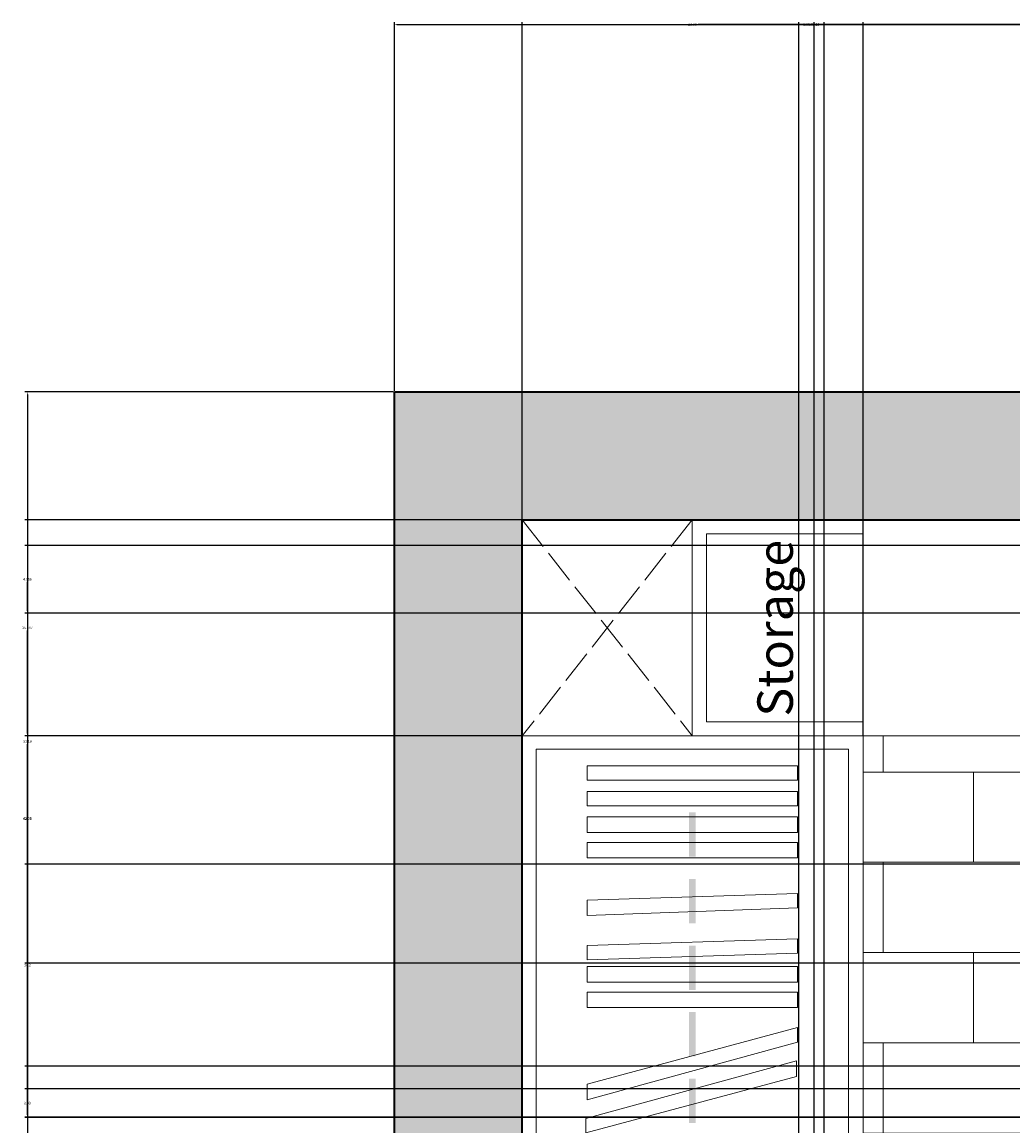
# Model space of a CAD drawing. Units: inches. Extents: x 6 to 575, y 34 to 566.
# Tile 8 of 21: x 6 to 76, y 488 to 566. Entities that reach past the tile are written whole.
import ezdxf

# ---------------------------------------------------------------- set-up
doc = ezdxf.new("R2010")
doc.units = ezdxf.units.IN
doc.linetypes.add('ACAD_ISO02W100', pattern=[15, 12, -3])
for name, color, linetype, lineweight in [('A-ANNO-DIMS', 2, 'Continuous', 18), ('A-ANNO-TEXT', 6, 'Continuous', 18), ('A-FLOR-CASE', 2, 'Continuous', 18), ('A-FLOR-CASE-HIDN', 2, 'ACAD_ISO02W100', 13), ('A-FLOR-PATT', 252, 'Continuous', 9), ('A-WALL-PATT', 251, 'Continuous', 9), ('WALLS', 7, 'Continuous', 35)]:
    doc.layers.add(name, color=color, linetype=linetype, lineweight=lineweight)
doc.styles.add('PDF Century Gothic', font='txt')
doc.styles.get("Standard").update_dxf_attribs({"font": 'arial.ttf'})
doc.dimstyles.get("Standard").update_dxf_attribs({"dimtxt": 0.18, "dimasz": 0.18, "dimexe": 0.18, "dimexo": 0.0625, "dimgap": 0.09, "dimtad": 0, "dimtih": 1, "dimtoh": 1, "dimdec": 4, "dimzin": 0, "dimdsep": 46, "dimtxsty": 'Standard', "dimcen": 0.09, "dimadec": 0, "dimazin": 0, "dimtfac": 1, "dimtdec": 4, "dimtofl": 0, "dimtmove": 0, "dimatfit": 3, "dimfxl": 1, "dimtolj": 1, "dimtzin": 0, "dimarcsym": 0})

# ---------------------------------------------------------------- blocks, each defined once
blk = doc.blocks.new('*D30')
at = {"layer": 'A-ANNO-DIMS', "color": 0, "lineweight": -2, "transparency": 16777216}
for p, q in [((32.596, 539.801), (6.649, 539.801)), ((6.829, 539.621), (6.829, 299.97)), ((6.829, 59.955), (6.829, 299.606)), ((197.625, 59.775), (6.649, 59.775))]:
    blk.add_line(p, q, dxfattribs=at)
at = {"layer": 'A-ANNO-DIMS', "color": 0, "transparency": 16777216}
for points in [[(6.799, 539.621), (6.859, 539.621), (6.829, 539.801)], [(6.799, 59.955), (6.859, 59.955), (6.829, 59.775)]]:
    blk.add_solid(points, dxfattribs=at)
at = {"layer": 'Defpoints', "color": 0, "transparency": 16777216}
for p in [(32.659, 539.801), (6.829, 59.775), (197.687, 59.775)]:
    blk.add_point(p, dxfattribs=at)
at = {"layer": 'A-ANNO-DIMS', "color": 0, "transparency": 16777216, "insert": (6.829, 299.788), "char_height": 0.18, "attachment_point": 5}
blk.add_mtext('\\A1;480', dxfattribs=at)
blk = doc.blocks.new('*D31')
at = {"layer": 'A-ANNO-DIMS', "color": 0, "lineweight": -2, "transparency": 16777216}
for p, q in [((32.659, 539.863), (32.659, 565.811)), ((32.839, 565.631), (96.378, 565.631)), ((160.479, 565.631), (96.939, 565.631)), ((160.659, 539.863), (160.659, 565.811))]:
    blk.add_line(p, q, dxfattribs=at)
at = {"layer": 'A-ANNO-DIMS', "color": 0, "transparency": 16777216}
for points in [[(32.839, 565.661), (32.839, 565.601), (32.659, 565.631)], [(160.479, 565.661), (160.479, 565.601), (160.659, 565.631)]]:
    blk.add_solid(points, dxfattribs=at)
at = {"layer": 'Defpoints', "color": 0, "transparency": 16777216}
for p in [(160.659, 565.631), (32.659, 539.801), (160.659, 539.801)]:
    blk.add_point(p, dxfattribs=at)
at = {"layer": 'A-ANNO-DIMS', "color": 0, "transparency": 16777216, "insert": (96.659, 565.631), "char_height": 0.18, "attachment_point": 5}
blk.add_mtext('\\A1;128', dxfattribs=at)
blk = doc.blocks.new('*D55')
at = {"layer": 'A-ANNO-DIMS', "color": 0, "lineweight": -2, "transparency": 16777216}
for p, q in [((41.659, 286.127), (41.659, 565.811)), ((41.839, 565.631), (81.788, 565.631)), ((122.385, 565.631), (82.436, 565.631)), ((122.565, 286.127), (122.565, 565.811))]:
    blk.add_line(p, q, dxfattribs=at)
at = {"layer": 'A-ANNO-DIMS', "color": 0, "transparency": 16777216}
for points in [[(41.839, 565.661), (41.839, 565.601), (41.659, 565.631)], [(122.385, 565.661), (122.385, 565.601), (122.565, 565.631)]]:
    blk.add_solid(points, dxfattribs=at)
at = {"layer": 'Defpoints', "color": 0, "transparency": 16777216}
for p in [(122.565, 565.631), (41.659, 286.064), (122.565, 286.064)]:
    blk.add_point(p, dxfattribs=at)
at = {"layer": 'A-ANNO-DIMS', "color": 0, "transparency": 16777216, "insert": (82.112, 565.631), "char_height": 0.18, "attachment_point": 5}
blk.add_mtext('\\A1;80.9', dxfattribs=at)
blk = doc.blocks.new('*D66')
at = {"layer": 'A-ANNO-DIMS', "color": 0, "lineweight": -2, "transparency": 16777216}
for p, q in [((41.659, 440.863), (41.659, 565.811)), ((41.839, 565.631), (61.878, 565.631)), ((82.712, 565.631), (62.673, 565.631)), ((82.892, 440.863), (82.892, 565.811))]:
    blk.add_line(p, q, dxfattribs=at)
at = {"layer": 'A-ANNO-DIMS', "color": 0, "transparency": 16777216}
for points in [[(41.839, 565.661), (41.839, 565.601), (41.659, 565.631)], [(82.712, 565.661), (82.712, 565.601), (82.892, 565.631)]]:
    blk.add_solid(points, dxfattribs=at)
at = {"layer": 'Defpoints', "color": 0, "transparency": 16777216}
for p in [(82.892, 565.631), (41.659, 440.801), (82.892, 440.801)]:
    blk.add_point(p, dxfattribs=at)
at = {"layer": 'A-ANNO-DIMS', "color": 0, "transparency": 16777216, "insert": (62.275, 565.631), "char_height": 0.18, "attachment_point": 5}
blk.add_mtext('\\A1;41.23', dxfattribs=at)
blk = doc.blocks.new('*D68')
at = {"layer": 'A-ANNO-DIMS', "color": 0, "lineweight": -2, "transparency": 16777216}
for p, q in [((206.596, 530.801), (6.649, 530.801)), ((6.829, 530.621), (6.829, 509.957)), ((6.829, 488.928), (6.829, 509.593)), ((248.571, 488.748), (6.649, 488.748))]:
    blk.add_line(p, q, dxfattribs=at)
at = {"layer": 'A-ANNO-DIMS', "color": 0, "transparency": 16777216}
for points in [[(6.799, 530.621), (6.859, 530.621), (6.829, 530.801)], [(6.799, 488.928), (6.859, 488.928), (6.829, 488.748)]]:
    blk.add_solid(points, dxfattribs=at)
at = {"layer": 'Defpoints', "color": 0, "transparency": 16777216}
for p in [(206.659, 530.801), (6.829, 488.748), (248.633, 488.748)]:
    blk.add_point(p, dxfattribs=at)
at = {"layer": 'A-ANNO-DIMS', "color": 0, "transparency": 16777216, "insert": (6.829, 509.775), "char_height": 0.18, "attachment_point": 5}
blk.add_mtext('\\A1;42.05', dxfattribs=at)
blk = doc.blocks.new('*D71')
at = {"layer": 'A-ANNO-DIMS', "color": 0, "lineweight": -2, "transparency": 16777216}
for p, q in [((246.62, 490.777), (6.649, 490.777)), ((6.829, 490.597), (6.829, 489.945)), ((6.829, 488.928), (6.829, 489.581)), ((248.571, 488.748), (6.649, 488.748))]:
    blk.add_line(p, q, dxfattribs=at)
at = {"layer": 'A-ANNO-DIMS', "color": 0, "transparency": 16777216}
for points in [[(6.799, 490.597), (6.859, 490.597), (6.829, 490.777)], [(6.799, 488.928), (6.859, 488.928), (6.829, 488.748)]]:
    blk.add_solid(points, dxfattribs=at)
at = {"layer": 'Defpoints', "color": 0, "transparency": 16777216}
for p in [(246.683, 490.777), (6.829, 488.748), (248.633, 488.748)]:
    blk.add_point(p, dxfattribs=at)
at = {"layer": 'A-ANNO-DIMS', "color": 0, "transparency": 16777216, "insert": (6.829, 489.763), "char_height": 0.18, "attachment_point": 5}
blk.add_mtext('\\A1;2.03', dxfattribs=at)
blk = doc.blocks.new('*D111')
at = {"layer": 'A-ANNO-DIMS', "color": 0, "lineweight": -2, "transparency": 16777216}
for p, q in [((41.659, 530.863), (41.659, 565.811)), ((41.839, 565.631), (53.259, 565.631)), ((65.469, 565.631), (54.049, 565.631)), ((65.649, 515.657), (65.649, 565.811))]:
    blk.add_line(p, q, dxfattribs=at)
at = {"layer": 'A-ANNO-DIMS', "color": 0, "transparency": 16777216}
for points in [[(41.839, 565.661), (41.839, 565.601), (41.659, 565.631)], [(65.469, 565.661), (65.469, 565.601), (65.649, 565.631)]]:
    blk.add_solid(points, dxfattribs=at)
at = {"layer": 'Defpoints', "color": 0, "transparency": 16777216}
for p in [(65.649, 565.631), (41.659, 530.801), (65.649, 515.594)]:
    blk.add_point(p, dxfattribs=at)
at = {"layer": 'A-ANNO-DIMS', "color": 0, "transparency": 16777216, "insert": (53.654, 565.631), "char_height": 0.18, "attachment_point": 5}
blk.add_mtext('\\A1;23.99', dxfattribs=at)
blk = doc.blocks.new('*D112')
at = {"layer": 'A-ANNO-DIMS', "color": 0, "lineweight": -2, "transparency": 16777216}
for p, q in [((41.596, 530.801), (6.649, 530.801)), ((6.829, 530.621), (6.829, 523.379)), ((6.829, 515.774), (6.829, 523.016)), ((41.596, 515.594), (6.649, 515.594))]:
    blk.add_line(p, q, dxfattribs=at)
at = {"layer": 'A-ANNO-DIMS', "color": 0, "transparency": 16777216}
for points in [[(6.799, 530.621), (6.859, 530.621), (6.829, 530.801)], [(6.799, 515.774), (6.859, 515.774), (6.829, 515.594)]]:
    blk.add_solid(points, dxfattribs=at)
at = {"layer": 'Defpoints', "color": 0, "transparency": 16777216}
for p in [(41.659, 530.801), (6.829, 515.594), (41.659, 515.594)]:
    blk.add_point(p, dxfattribs=at)
at = {"layer": 'A-ANNO-DIMS', "color": 0, "transparency": 16777216, "insert": (6.829, 523.198), "char_height": 0.18, "attachment_point": 5}
blk.add_mtext('\\A1;15.207', dxfattribs=at)
blk = doc.blocks.new('*D113')
at = {"layer": 'A-ANNO-DIMS', "color": 0, "lineweight": -2, "transparency": 16777216}
for p, q in [((65.649, 530.863), (65.649, 565.811)), ((65.829, 565.631), (91.278, 565.631)), ((117.479, 565.631), (92.03, 565.631)), ((117.659, 530.863), (117.659, 565.811))]:
    blk.add_line(p, q, dxfattribs=at)
at = {"layer": 'A-ANNO-DIMS', "color": 0, "transparency": 16777216}
for points in [[(65.829, 565.661), (65.829, 565.601), (65.649, 565.631)], [(117.479, 565.661), (117.479, 565.601), (117.659, 565.631)]]:
    blk.add_solid(points, dxfattribs=at)
at = {"layer": 'Defpoints', "color": 0, "transparency": 16777216}
for p in [(117.659, 565.631), (65.649, 530.801), (117.659, 530.801)]:
    blk.add_point(p, dxfattribs=at)
at = {"layer": 'A-ANNO-DIMS', "color": 0, "transparency": 16777216, "insert": (91.654, 565.631), "char_height": 0.18, "attachment_point": 5}
blk.add_mtext('\\A1;52.01', dxfattribs=at)
blk = doc.blocks.new('*D115')
at = {"layer": 'A-ANNO-DIMS', "color": 0, "lineweight": -2, "transparency": 16777216}
for p, q in [((60.944, 565.631), (60.764, 565.631)), ((61.124, 427.26), (61.124, 565.811)), ((62.217, 427.26), (62.217, 565.811)), ((62.397, 565.631), (62.577, 565.631))]:
    blk.add_line(p, q, dxfattribs=at)
at = {"layer": 'A-ANNO-DIMS', "color": 0, "transparency": 16777216}
for points in [[(60.944, 565.661), (60.944, 565.601), (61.124, 565.631)], [(62.397, 565.661), (62.397, 565.601), (62.217, 565.631)]]:
    blk.add_solid(points, dxfattribs=at)
at = {"layer": 'Defpoints', "color": 0, "transparency": 16777216}
for p in [(62.217, 565.631), (61.124, 427.198), (62.217, 427.198)]:
    blk.add_point(p, dxfattribs=at)
at = {"layer": 'A-ANNO-DIMS', "color": 0, "transparency": 16777216, "insert": (61.67, 565.631), "char_height": 0.18, "attachment_point": 5}
blk.add_mtext('\\A1;1.09', dxfattribs=at)
blk = doc.blocks.new('*D116')
at = {"layer": 'A-ANNO-DIMS', "color": 0, "lineweight": -2, "transparency": 16777216}
for p, q in [((61.124, 427.26), (61.124, 565.811)), ((61.304, 565.631), (61.706, 565.631)), ((62.739, 565.631), (62.337, 565.631)), ((62.919, 427.26), (62.919, 565.811))]:
    blk.add_line(p, q, dxfattribs=at)
at = {"layer": 'A-ANNO-DIMS', "color": 0, "transparency": 16777216}
for points in [[(61.304, 565.661), (61.304, 565.601), (61.124, 565.631)], [(62.739, 565.661), (62.739, 565.601), (62.919, 565.631)]]:
    blk.add_solid(points, dxfattribs=at)
at = {"layer": 'Defpoints', "color": 0, "transparency": 16777216}
for p in [(62.919, 565.631), (61.124, 427.198), (62.919, 427.198)]:
    blk.add_point(p, dxfattribs=at)
at = {"layer": 'A-ANNO-DIMS', "color": 0, "transparency": 16777216, "insert": (62.022, 565.631), "char_height": 0.18, "attachment_point": 5}
blk.add_mtext('\\A1;1.79', dxfattribs=at)
blk = doc.blocks.new('*D117')
at = {"layer": 'A-ANNO-DIMS', "color": 0, "lineweight": -2, "transparency": 16777216}
for p, q in [((41.596, 515.594), (6.649, 515.594)), ((6.829, 515.414), (6.829, 478.379)), ((6.829, 440.981), (6.829, 478.016)), ((41.596, 440.801), (6.649, 440.801))]:
    blk.add_line(p, q, dxfattribs=at)
at = {"layer": 'A-ANNO-DIMS', "color": 0, "transparency": 16777216}
for points in [[(6.799, 515.414), (6.859, 515.414), (6.829, 515.594)], [(6.799, 440.981), (6.859, 440.981), (6.829, 440.801)]]:
    blk.add_solid(points, dxfattribs=at)
at = {"layer": 'Defpoints', "color": 0, "transparency": 16777216}
for p in [(6.829, 515.594), (41.659, 515.594), (41.659, 440.801)]:
    blk.add_point(p, dxfattribs=at)
at = {"layer": 'A-ANNO-DIMS', "color": 0, "transparency": 16777216, "insert": (6.829, 478.198), "char_height": 0.18, "attachment_point": 5}
blk.add_mtext('\\A1;74.8', dxfattribs=at)
blk = doc.blocks.new('*D118')
at = {"layer": 'A-ANNO-DIMS', "color": 0, "lineweight": -2, "transparency": 16777216}
for p, q in [((65.649, 515.657), (65.649, 565.811)), ((65.829, 565.631), (78.186, 565.631)), ((91.474, 565.631), (79.118, 565.631)), ((91.654, 515.657), (91.654, 565.811))]:
    blk.add_line(p, q, dxfattribs=at)
at = {"layer": 'A-ANNO-DIMS', "color": 0, "transparency": 16777216}
for points in [[(65.829, 565.661), (65.829, 565.601), (65.649, 565.631)], [(91.474, 565.661), (91.474, 565.601), (91.654, 565.631)]]:
    blk.add_solid(points, dxfattribs=at)
at = {"layer": 'Defpoints', "color": 0, "transparency": 16777216}
for p in [(91.654, 565.631), (65.649, 515.594), (91.654, 515.594)]:
    blk.add_point(p, dxfattribs=at)
at = {"layer": 'A-ANNO-DIMS', "color": 0, "transparency": 16777216, "insert": (78.652, 565.631), "char_height": 0.18, "attachment_point": 5}
blk.add_mtext('\\A1;26.005', dxfattribs=at)
blk = doc.blocks.new('*D176')
at = {"layer": 'A-ANNO-DIMS', "color": 0, "lineweight": -2, "transparency": 16777216}
for p, q in [((121.596, 530.801), (6.649, 530.801)), ((6.829, 530.621), (6.829, 509.974)), ((6.829, 488.963), (6.829, 509.61)), ((121.839, 488.783), (6.649, 488.783))]:
    blk.add_line(p, q, dxfattribs=at)
at = {"layer": 'A-ANNO-DIMS', "color": 0, "transparency": 16777216}
for points in [[(6.799, 530.621), (6.859, 530.621), (6.829, 530.801)], [(6.799, 488.963), (6.859, 488.963), (6.829, 488.783)]]:
    blk.add_solid(points, dxfattribs=at)
at = {"layer": 'Defpoints', "color": 0, "transparency": 16777216}
for p in [(121.659, 530.801), (6.829, 488.783), (121.902, 488.783)]:
    blk.add_point(p, dxfattribs=at)
at = {"layer": 'A-ANNO-DIMS', "color": 0, "transparency": 16777216, "insert": (6.829, 509.792), "char_height": 0.18, "attachment_point": 5}
blk.add_mtext('\\A1;42.02', dxfattribs=at)
blk = doc.blocks.new('*D177')
at = {"layer": 'A-ANNO-DIMS', "color": 0, "lineweight": -2, "transparency": 16777216}
for p, q in [((139.252, 528.983), (6.649, 528.983)), ((6.829, 528.803), (6.829, 526.786)), ((6.829, 524.404), (6.829, 526.422)), ((139.252, 524.224), (6.649, 524.224))]:
    blk.add_line(p, q, dxfattribs=at)
at = {"layer": 'A-ANNO-DIMS', "color": 0, "transparency": 16777216}
for points in [[(6.799, 528.803), (6.859, 528.803), (6.829, 528.983)], [(6.799, 524.404), (6.859, 524.404), (6.829, 524.224)]]:
    blk.add_solid(points, dxfattribs=at)
at = {"layer": 'Defpoints', "color": 0, "transparency": 16777216}
for p in [(139.314, 528.983), (6.829, 524.224), (139.314, 524.224)]:
    blk.add_point(p, dxfattribs=at)
at = {"layer": 'A-ANNO-DIMS', "color": 0, "transparency": 16777216, "insert": (6.829, 526.604), "char_height": 0.18, "attachment_point": 5}
blk.add_mtext('\\A1;4.759', dxfattribs=at)
blk = doc.blocks.new('*D181')
at = {"layer": 'A-ANNO-DIMS', "color": 0, "lineweight": -2, "transparency": 16777216}
for p, q in [((197.596, 530.801), (6.649, 530.801)), ((6.829, 530.621), (6.829, 515.387)), ((6.829, 499.788), (6.829, 515.023)), ((170.657, 499.608), (6.649, 499.608))]:
    blk.add_line(p, q, dxfattribs=at)
at = {"layer": 'A-ANNO-DIMS', "color": 0, "transparency": 16777216}
for points in [[(6.799, 530.621), (6.859, 530.621), (6.829, 530.801)], [(6.799, 499.788), (6.859, 499.788), (6.829, 499.608)]]:
    blk.add_solid(points, dxfattribs=at)
at = {"layer": 'Defpoints', "color": 0, "transparency": 16777216}
for p in [(197.659, 530.801), (6.829, 499.608), (170.719, 499.608)]:
    blk.add_point(p, dxfattribs=at)
at = {"layer": 'A-ANNO-DIMS', "color": 0, "transparency": 16777216, "insert": (6.829, 515.205), "char_height": 0.18, "attachment_point": 5}
blk.add_mtext('\\A1;31.19', dxfattribs=at)
blk = doc.blocks.new('*D183')
at = {"layer": 'A-ANNO-DIMS', "color": 0, "lineweight": -2, "transparency": 16777216}
for p, q in [((181.056, 506.572), (6.649, 506.572)), ((6.829, 506.392), (6.829, 499.652)), ((6.829, 492.552), (6.829, 499.291)), ((180.432, 492.372), (6.649, 492.372))]:
    blk.add_line(p, q, dxfattribs=at)
at = {"layer": 'A-ANNO-DIMS', "color": 0, "transparency": 16777216}
for points in [[(6.799, 506.392), (6.859, 506.392), (6.829, 506.572)], [(6.799, 492.552), (6.859, 492.552), (6.829, 492.372)]]:
    blk.add_solid(points, dxfattribs=at)
at = {"layer": 'Defpoints', "color": 0, "transparency": 16777216}
for p in [(6.829, 506.572), (181.118, 506.572), (180.494, 492.372)]:
    blk.add_point(p, dxfattribs=at)
at = {"layer": 'A-ANNO-DIMS', "color": 0, "transparency": 16777216, "insert": (6.829, 499.472), "char_height": 0.18, "attachment_point": 5}
blk.add_mtext('\\A1;14.2', dxfattribs=at)

msp = doc.modelspace()

# ---------------------------------------------------------------- hatches: boundary and pattern name
at = {"layer": 'A-FLOR-PATT'}
h = msp.add_hatch(dxfattribs=at)
h.set_pattern_fill('BRICK', color=256)
h.set_pattern_definition([(0, (-98.035, 170.1465), (0, 6.35), []), (90, (-98.035, 170.147), (-12.7, 8e-16), [6.35, -6.35]), (90, (-91.685, 170.147), (-12.7, 8e-16), [-6.35, 6.35])])
h.paths.add_polyline_path([(180.8711, 269.7588), (182.4439, 270.6668), (182.4628, 270.6341, -0.1161983), (201.8275, 275.5902), (201.8275, 276.801), (197.6586, 276.801), (197.6586, 293.1641), (182.6401, 293.1641), (182.6401, 348.324), (197.6586, 348.324), (197.6586, 407.7709), (112.8513, 407.7709), (112.8513, 431.801), (111.6586, 431.801), (111.6586, 440.801), (117.6586, 440.801), (117.6586, 446.801), (117.6586, 448.2751), (117.6586, 473.3269), (117.6586, 474.801), (117.6586, 515.5941), (100.2533, 515.5941, -1), (83.0548, 515.5941), (65.6494, 515.5941), (65.6494, 440.801), (82.8918, 440.801), (82.8918, 431.801), (82.8918, 407.7709), (41.6586, 407.7709), (41.6586, 379.0637), (62.6459, 379.0637), (62.6459, 358.0764), (122.565, 358.0764), (122.565, 286.0643), (62.6459, 286.0643), (62.6459, 265.077), (41.6586, 265.077), (41.6586, 224.801), (41.6586, 212.801), (71.6586, 212.801), (167.6586, 212.801), (197.6586, 212.801), (197.6586, 230.801), (201.8157, 230.801), (201.8157, 233.4817)])
h.paths.add_polyline_path([(133.3414, 245.1275), (133.3317, 245.1352), (133.3317, 245.104)], flags=16)
h.paths.add_polyline_path([(133.3317, 222.1662), (85.3496, 222.1662), (85.3496, 243.7443, -0.5009073), (87.1831, 246.1963), (107.4292, 246.1963), (111.2522, 246.1963), (131.4202, 246.1963, -0.4142136), (133.3317, 244.2848)], flags=16)
h.paths.add_polyline_path([(72.7105, 244.4018), (72.7105, 220.3718), (48.6804, 220.3718), (48.6804, 244.4018)], flags=16)
h.paths.add_polyline_path([(71.7466, 237.8955, -1), (59.8096, 237.8955, -1)], flags=0)
at = {"layer": 'A-WALL-PATT'}
h = msp.add_hatch(color=256, dxfattribs=at)
h.dxf.hatch_style = 1
h.paths.add_polyline_path([(160.6586, 539.801), (32.6586, 539.801), (32.6586, 272.801), (41.6586, 272.801), (41.6586, 286.0643), (41.6586, 358.0764), (41.6586, 379.0637), (41.6586, 407.7709), (41.6194, 407.7709), (41.6194, 431.801), (82.8918, 431.801), (82.8918, 440.801), (65.6494, 440.801), (65.6494, 440.7732), (41.6194, 440.7732), (41.6194, 515.5941), (41.6586, 530.801), (117.6586, 530.801), (117.6586, 474.801), (120.6068, 474.801), (121.6586, 474.801), (121.6586, 530.801), (137.4275, 530.801), (137.4275, 530.8356), (141.2505, 530.8356), (160.6586, 530.801)])
h.paths.add_polyline_path([(71.6586, 212.801), (41.6586, 212.801), (41.6586, 224.801), (32.6586, 224.801), (32.6586, 203.801), (71.6586, 203.801)])
h.paths.add_polyline_path([(206.6586, 215.801), (246.6586, 215.801), (246.6586, 224.801), (206.6586, 224.801), (206.6586, 230.801), (201.8157, 230.801), (197.6586, 230.801), (197.6586, 212.801), (167.6586, 212.801), (167.6586, 203.801), (206.6586, 203.801)])
h.paths.add_polyline_path([(383.6586, 224.801), (334.6586, 224.801), (334.6586, 215.801), (374.6586, 215.801), (374.6586, 203.801), (384.0753, 203.801), (407.6586, 203.801), (407.6586, 212.801), (383.6586, 212.801)])
h.paths.add_polyline_path([(548.6586, 270.801), (539.6586, 270.801), (539.6586, 212.801), (515.6586, 212.801), (515.6586, 203.801), (548.6586, 203.801)])
h.paths.add_polyline_path([(548.6586, 412.801), (545.7108, 412.801), (539.6586, 412.801), (539.6586, 382.801), (433.708, 382.801), (433.708, 378.801), (539.6586, 378.801), (539.6586, 366.801), (548.6586, 366.801)])
h.paths.add_polyline_path([(548.6586, 539.801), (455.9436, 539.801), (455.9436, 530.801), (539.6586, 530.801), (539.6586, 440.801), (548.6586, 440.801)])
h.paths.add_polyline_path([(407.9436, 539.801), (362.6586, 539.801), (362.6586, 530.801), (374.6586, 530.801), (374.6586, 452.801), (354.6586, 452.801), (354.6586, 448.801), (374.6586, 448.801), (374.6586, 278.801), (383.6586, 278.801), (383.6586, 530.801), (407.9436, 530.801)])
h.paths.add_polyline_path([(338.6586, 539.801), (320.6586, 539.801), (320.6586, 530.801), (322.6586, 530.801), (322.6586, 448.801), (326.6586, 448.801), (326.6586, 530.801), (338.6586, 530.801)])
h.paths.add_polyline_path([(272.6586, 539.801), (184.6586, 539.801), (184.6586, 530.801), (197.6586, 530.801), (197.6586, 440.801), (176.6714, 440.801), (121.6586, 440.801), (121.6586, 446.801), (117.6586, 446.801), (117.6586, 440.801), (111.6586, 440.801), (111.6586, 431.801), (197.6586, 431.801), (197.6586, 407.7709), (197.6586, 276.801), (206.6586, 276.801), (206.6586, 530.801), (272.6586, 530.801)])

# ---------------------------------------------------------------- linework, layer by layer
at = {"layer": 'A-FLOR-CASE'}
for p, q in [((53.6344, 515.5941), (53.6344, 530.801)), ((65.6494, 515.5941), (65.6494, 530.801)), ((65.6494, 529.801), (54.6344, 529.801)), ((54.6344, 516.5941), (54.6344, 529.801)), ((65.6494, 516.5941), (54.6344, 516.5941)), ((41.6194, 515.5941), (117.6586, 515.5941))]:
    msp.add_line(p, q, dxfattribs=at)
for points in [[(41.6194, 515.5941), (41.6194, 440.7732), (65.6494, 440.7732), (65.6494, 515.5941)], [(42.6336, 514.6578), (42.6336, 441.7875), (64.6352, 441.7875), (64.6352, 514.6578)], [(46.2226, 513.4875), (61.0463, 513.4875), (61.0463, 512.4733), (46.2226, 512.4733)], [(46.2226, 511.6931), (61.0463, 511.6931), (61.0463, 510.6788), (46.2226, 510.6788)], [(46.2226, 509.8986), (61.0463, 509.8986), (61.0463, 508.8064), (46.2226, 508.8064)], [(46.2226, 508.1042), (61.0463, 508.1042), (61.0463, 507.0119), (46.2226, 507.0119)], [(46.2226, 504.0472), (61.0463, 504.5153), (61.0463, 503.501), (46.2226, 502.9549)], [(46.2226, 500.8484), (61.0463, 501.3165), (61.0463, 500.3022), (46.2226, 499.8341)], [(46.2226, 499.366), (61.0463, 499.366), (61.0463, 498.2737), (46.2226, 498.2737)], [(46.2226, 497.5715), (61.0463, 497.5715), (61.0463, 496.4793), (46.2226, 496.4793)], [(46.2226, 490.0036), (61.0463, 494.0606), (61.0463, 495.0749), (46.2226, 491.0959)], [(46.1445, 487.663), (60.9683, 491.642), (60.9683, 492.7343), (46.1445, 488.6773)]]:
    msp.add_lwpolyline(points, close=True, dxfattribs=at)
at = {"layer": 'A-FLOR-CASE', "transparency": 33554559}
for points in [[(53.4004, 507.0899), (53.8685, 507.0899), (53.4004, 510.2107)], [(53.8685, 507.0899), (53.4004, 510.2107), (53.8685, 510.2107)], [(53.4004, 502.4087), (53.8685, 502.4087), (53.4004, 505.5295)], [(53.8685, 502.4087), (53.4004, 505.5295), (53.8685, 505.5295)], [(53.4004, 497.7276), (53.8685, 497.7276), (53.4004, 500.8484)], [(53.8685, 497.7276), (53.4004, 500.8484), (53.8685, 500.8484)], [(53.4004, 493.0464), (53.8685, 493.0464), (53.4004, 496.1672)], [(53.8685, 493.0464), (53.4004, 496.1672), (53.8685, 496.1672)], [(53.4004, 488.3652), (53.8685, 488.3652), (53.4004, 491.486)], [(53.8685, 488.3652), (53.4004, 491.486), (53.8685, 491.486)]]:
    msp.add_solid(points, dxfattribs=at)
at = {"layer": 'A-FLOR-CASE-HIDN', "ltscale": 0.2}
for p, q in [((53.6344, 530.801), (41.6586, 515.5941)), ((41.6586, 530.801), (53.6344, 515.5941))]:
    msp.add_line(p, q, dxfattribs=at)
at = {"layer": 'WALLS'}
for p, q in [((32.6586, 539.801), (32.6586, 539.801)), ((32.6586, 539.801), (160.6586, 539.801)), ((32.6586, 272.801), (32.6586, 539.801)), ((41.6586, 530.801), (117.6586, 530.801)), ((41.6586, 440.801), (41.6586, 530.801))]:
    msp.add_line(p, q, dxfattribs=at)

# ---------------------------------------------------------------- texts
at = {"layer": 'A-ANNO-TEXT', "insert": (59.7859, 516.946), "char_height": 2.50021, "attachment_point": 4, "rotation": 90, "style": 'PDF Century Gothic'}
msp.add_mtext('Storage', dxfattribs=at)

# ---------------------------------------------------------------- dimensions: what is measured, and where the dimension line sits
at = {"layer": 'A-ANNO-DIMS'}
for base, p1, p2, override, picture, middle in [((160.6586, 565.631), (32.6586, 539.801), (160.6586, 539.801), {"dimdec": 0, "dimlfac": 1, "dimrnd": 0, "dimzin": 0, "dimdsep": 46, "dimlunit": 2}, '*D31', (96.6586, 565.631)), ((122.565, 565.631), (41.6586, 286.0643), (122.565, 286.0643), {"dimdec": 1, "dimlfac": 1, "dimrnd": 0, "dimzin": 0, "dimdsep": 46, "dimlunit": 2}, '*D55', (82.1118, 565.631)), ((82.8918, 565.631), (41.6586, 440.801), (82.8918, 440.801), {"dimdec": 2, "dimlfac": 1, "dimrnd": 0, "dimzin": 0, "dimdsep": 46, "dimlunit": 2}, '*D66', (62.2752, 565.631)), ((65.6494, 565.631), (41.6586, 530.801), (65.6494, 515.5941), {"dimdec": 2, "dimlfac": 1, "dimrnd": 0, "dimzin": 0, "dimdsep": 46, "dimlunit": 2}, '*D111', (53.654, 565.631)), ((62.2166, 565.631), (61.1243, 427.1978), (62.2166, 427.1978), {"dimdec": 2, "dimlfac": 1, "dimrnd": 0, "dimzin": 0, "dimdsep": 46, "dimlunit": 2}, '*D115', (61.6704, 565.631)), ((62.9188, 565.631), (61.1243, 427.1978), (62.9188, 427.1978), {"dimdec": 2, "dimlfac": 1, "dimrnd": 0, "dimzin": 0, "dimdsep": 46, "dimlunit": 2}, '*D116', (62.0215, 565.631)), ((117.6586, 565.631), (65.6494, 530.801), (117.6586, 530.801), {"dimdec": 2, "dimlfac": 1, "dimrnd": 0, "dimzin": 0, "dimdsep": 46, "dimlunit": 2}, '*D113', (91.654, 565.631)), ((91.654, 565.631), (65.6494, 515.5941), (91.654, 515.5941), {"dimdec": 3, "dimlfac": 1, "dimrnd": 0, "dimzin": 0, "dimdsep": 46, "dimlunit": 2}, '*D118', (78.6517, 565.631))]:
    dim = msp.add_linear_dim(base=base, p1=p1, p2=p2, dimstyle='Standard', override=override, dxfattribs=at)
    dim.commit()
    dim.dimension.update_dxf_attribs({"geometry": picture, "text_midpoint": middle})
for base, p1, p2, override, picture, middle in [((6.8286, 59.7747), (32.6586, 539.801), (197.6872, 59.7747), {"dimdec": 0, "dimlfac": 1, "dimrnd": 0, "dimzin": 0, "dimdsep": 46, "dimlunit": 2}, '*D30', (6.8286, 299.7878)), ((6.8286, 515.5941), (41.6586, 530.801), (41.6586, 515.5941), {"dimdec": 3, "dimlfac": 1, "dimrnd": 0, "dimzin": 0, "dimdsep": 46, "dimlunit": 2}, '*D112', (6.8286, 523.1975)), ((6.8286, 488.7484), (206.6586, 530.801), (248.6332, 488.7484), {"dimdec": 2, "dimlfac": 1, "dimrnd": 0, "dimzin": 0, "dimdsep": 46, "dimlunit": 2}, '*D68', (6.8286, 509.7747)), ((6.8286, 488.7831), (121.6586, 530.801), (121.9016, 488.7831), {"dimdec": 2, "dimlfac": 1, "dimrnd": 0, "dimzin": 0, "dimdsep": 46, "dimlunit": 2}, '*D176', (6.8286, 509.792)), ((6.8286, 499.6084), (197.6586, 530.801), (170.7195, 499.6084), {"dimdec": 2, "dimlfac": 1, "dimrnd": 0, "dimzin": 0, "dimdsep": 46, "dimlunit": 2}, '*D181', (6.8286, 515.2047)), ((6.8286, 524.224), (139.3143, 528.9833), (139.3143, 524.224), {"dimdec": 3, "dimlfac": 1, "dimrnd": 0, "dimzin": 0, "dimdsep": 46, "dimlunit": 2}, '*D177', (6.8286, 526.6036)), ((6.8286, 515.5941), (41.6586, 440.801), (41.6586, 515.5941), {"dimdec": 1, "dimlfac": 1, "dimrnd": 0, "dimzin": 0, "dimdsep": 46, "dimlunit": 2}, '*D117', (6.8286, 478.1975)), ((6.8286, 506.5715), (180.4943, 492.372), (181.1185, 506.5715), {"dimdec": 1, "dimlfac": 1, "dimrnd": 0, "dimzin": 0, "dimdsep": 46, "dimlunit": 2}, '*D183', (6.8286, 499.4717)), ((6.8286, 488.7484), (246.6827, 490.7769), (248.6332, 488.7484), {"dimdec": 2, "dimlfac": 1, "dimrnd": 0, "dimzin": 0, "dimdsep": 46, "dimlunit": 2}, '*D71', (6.8286, 489.7627))]:
    dim = msp.add_linear_dim(base=base, p1=p1, p2=p2, angle=90, dimstyle='Standard', override=override, dxfattribs=at)
    dim.commit()
    dim.dimension.update_dxf_attribs({"geometry": picture, "text_midpoint": middle})

doc.saveas('drawing.dxf')
